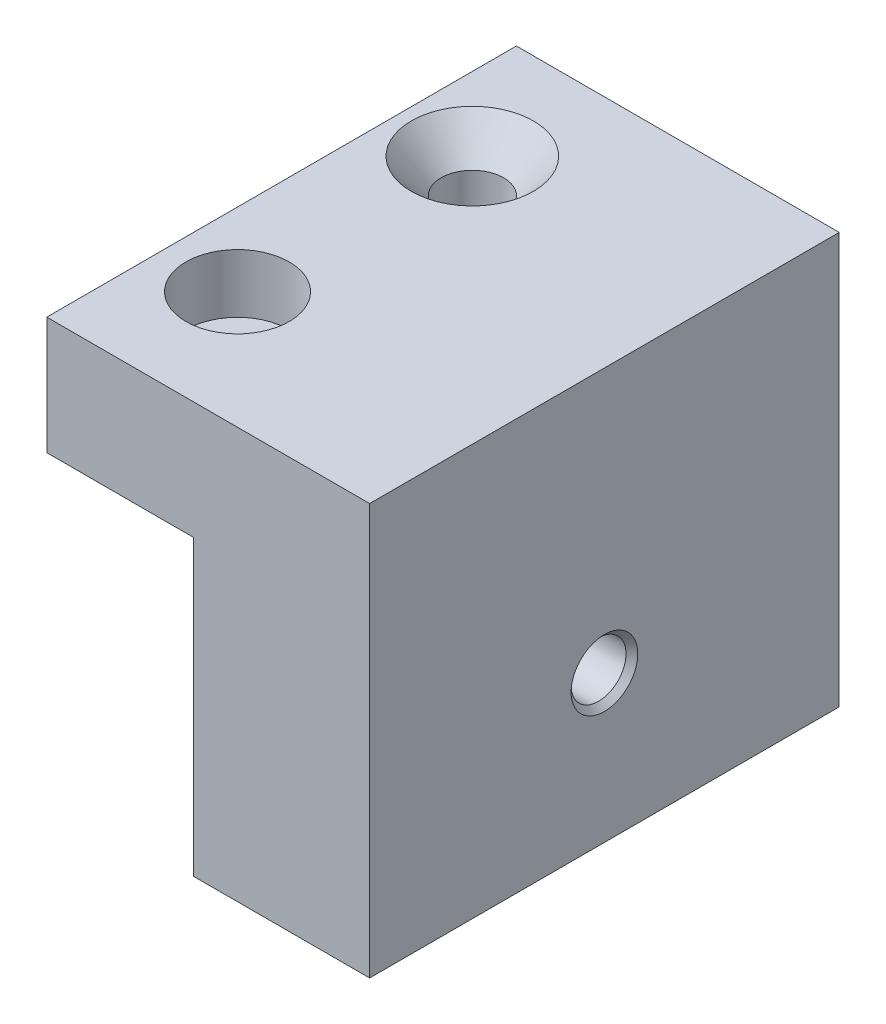
from build123d import *

# Parameters (mm, degrees)
BLOCK_BODY_2IN_DEPTH                      = 50.8
SIDE_THROUGH_HOLE_0_234_D                 = 5.9436
SIDE_HOLE_EDGE_CHAMFER_SIZE               = 0.635
DOWEL_HOLE_0_126_D                        = 3.2004
DOWEL_HOLE_0_126_DEPTH                    = 6.0198
DOWEL_HOLE_0_126_TIP                      = 1.6002
COUNTERSUNK_SCREW_HOLE_NO0_D              = 6.7564
COUNTERSUNK_SCREW_HOLE_NO0_CSINK_D        = 13.208
COUNTERSUNK_SCREW_HOLE_NO0_CSINK_ANGLE    = 82
COUNTERBORED_BOLT_HOLE_0_25IN_D           = 6.7564
COUNTERBORED_BOLT_HOLE_0_25IN_CBORE_D     = 11.176
COUNTERBORED_BOLT_HOLE_0_25IN_CBORE_DEPTH = 6.35


with BuildPart() as part:
    # Block Profile Sketch → Block Body 2in (new body)
    with BuildSketch(Plane.XY):
        Polygon((0, 12.7), (19.05, 12.7), (19.05, -31.75), (0, -31.75), (0, 0), (-15.875, 0), (-15.875, 12.7), align=None)
    extrude(amount=BLOCK_BODY_2IN_DEPTH)

    # Side Through Hole Ø0.234 (through all)
    with Locations(Plane(origin=(0, -15.875, 25.4), x_dir=(0, -1, 0), z_dir=(-1, 0, 0))):
        with Locations((0, 0)):
            Hole(SIDE_THROUGH_HOLE_0_234_D / 2)

    # Side Hole Edge Chamfer
    side_hole_edge_chamfer_edges = [part.edges().sort_by_distance(p)[0] for p in [
        (0, -18.8468, 25.4),
        (19.05, -18.8468, 25.4),
    ]]
    chamfer(side_hole_edge_chamfer_edges, length=SIDE_HOLE_EDGE_CHAMFER_SIZE)

    # Dowel Hole Ø0.126
    with Locations(Plane(origin=(-7.9375, 0, 25.4), x_dir=(-1, 0, 0), z_dir=(0, -1, 0))):
        with Locations((0, 0)):
            Hole(DOWEL_HOLE_0_126_D / 2, depth=DOWEL_HOLE_0_126_DEPTH)
            with Locations((0, 0, -(DOWEL_HOLE_0_126_DEPTH + DOWEL_HOLE_0_126_TIP / 2))):  # 90° drill point
                Cone(0, DOWEL_HOLE_0_126_D / 2, DOWEL_HOLE_0_126_TIP, mode=Mode.SUBTRACT)

    # Countersunk Screw Hole No0 (through all)
    with Locations(Plane(origin=(-7.9375, 12.7, 12.7), x_dir=(0, 0, 1), z_dir=(0, 1, 0))):
        with Locations((0, 0)):
            CounterSinkHole(COUNTERSUNK_SCREW_HOLE_NO0_D / 2, COUNTERSUNK_SCREW_HOLE_NO0_CSINK_D / 2, counter_sink_angle=COUNTERSUNK_SCREW_HOLE_NO0_CSINK_ANGLE)

    # Counterbored Bolt Hole 0.25in (through all)
    with Locations(Plane(origin=(-7.9375, 12.7, 38.1), x_dir=(0, 0, 1), z_dir=(0, 1, 0))):
        with Locations((0, 0)):
            CounterBoreHole(COUNTERBORED_BOLT_HOLE_0_25IN_D / 2, COUNTERBORED_BOLT_HOLE_0_25IN_CBORE_D / 2, COUNTERBORED_BOLT_HOLE_0_25IN_CBORE_DEPTH)


solid = part.part
